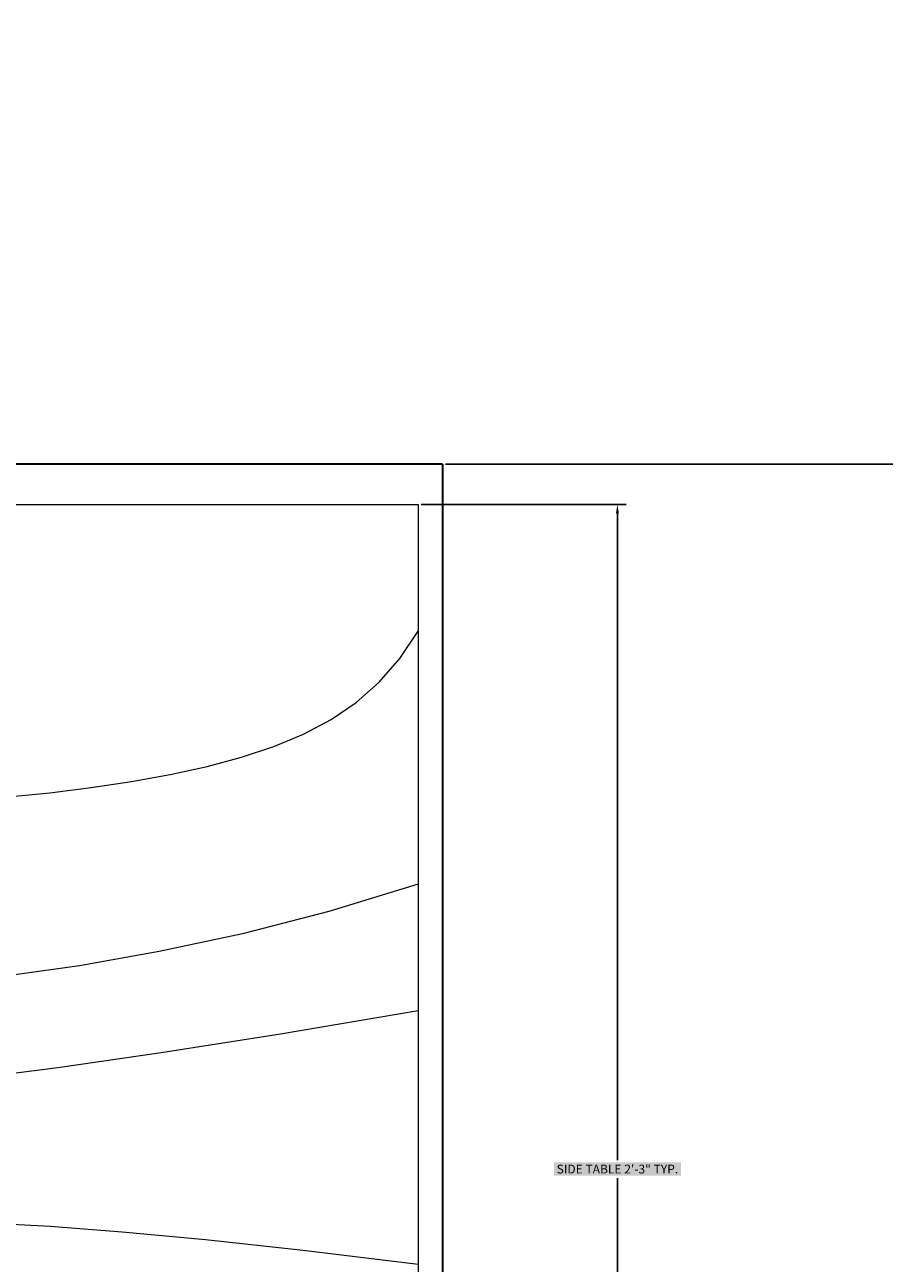
# Model space of a CAD drawing. Units: inches. Extents: x -128 to 854, y -395 to 398.
# Tile 41 of 61: x 296 to 314, y 170 to 196. Entities that reach past the tile are written whole.
import ezdxf

# ---------------------------------------------------------------- set-up
doc = ezdxf.new("R2010")
doc.units = ezdxf.units.IN
doc.header["$MEASUREMENT"] = 0
for name, color, linetype, lineweight in [('A-ANNO-DIMS', 2, 'Continuous', 18), ('A-FURN', 8, 'Continuous', 18), ('A-WALL', 4, 'Continuous', 35)]:
    doc.layers.add(name, color=color, linetype=linetype, lineweight=lineweight)
doc.styles.get("Standard").update_dxf_attribs({"font": 'arial.ttf'})
doc.dimstyles.get("Standard").update_dxf_attribs({"dimtxt": 0.18, "dimasz": 0.18, "dimexe": 0.18, "dimexo": 0.0625, "dimgap": 0.09, "dimtad": 0, "dimtih": 1, "dimtoh": 1, "dimdec": 1, "dimzin": 0, "dimdsep": 46, "dimlunit": 4, "dimtxsty": 'Standard', "dimcen": 0.09, "dimclrd": 1, "dimclre": 2, "dimclrt": 6, "dimadec": 0, "dimazin": 0, "dimtfac": 1, "dimtdec": 1, "dimtofl": 0, "dimtmove": 0, "dimatfit": 3, "dimfxl": 1, "dimtfill": 2, "dimtfillclr": 3, "dimtolj": 1, "dimtzin": 0, "dimarcsym": 0})

# ---------------------------------------------------------------- blocks, each defined once
blk = doc.blocks.new('Table - Square Woodgrain 42 x 42 in.')
for points in [[(0, -42), (0, 0), (42, 0), (42, -42)], [(29.0383, -9.2382), (30.3655, -9.1068), (31.6728, -8.9455), (32.9461, -8.7535), (34.1717, -8.5304), (35.3358, -8.2756), (36.4268, -7.9863), (37.443, -7.6521), (38.3849, -7.2603), (39.253, -6.7986), (40.048, -6.2542), (40.7705, -5.6147), (41.421, -4.8674), (42, -4)], [(42, -12), (39.1784, -12.8621), (36.4519, -13.5654), (33.8246, -14.1294), (31.3004, -14.5731), (28.8832, -14.9161)], [(42, -16), (37.6529, -16.7365), (33.8802, -17.329), (30.6179, -17.7961), (27.8015, -18.1561)], [(0, -24), (3.9243, -23.6805), (7.4766, -23.4138), (10.6891, -23.1954), (13.5943, -23.0205), (16.2247, -22.8847), (18.6125, -22.7832), (20.7903, -22.7116), (22.7903, -22.6651), (24.6563, -22.642), (26.4764, -22.6507), (28.35, -22.7024), (30.3766, -22.8084), (32.6555, -22.98), (35.2861, -23.2283), (38.3678, -23.5645), (42, -24)]]:
    blk.add_lwpolyline(points)
blk = doc.blocks.new('*D55')
at = {"layer": 'A-ANNO-DIMS', "color": 0, "lineweight": -2, "transparency": 16777216}
for p, q in [((304.81, 186.741), (221.092, 186.741)), ((221.272, 181.741), (221.272, 131.873)), ((221.272, 77.741), (221.272, 127.608)), ((304.81, 72.741), (221.092, 72.741))]:
    blk.add_line(p, q, dxfattribs=at)
at = {"layer": 'A-ANNO-DIMS', "color": 0, "transparency": 16777216}
for points in [[(220.439, 181.741), (222.105, 181.741), (221.272, 186.741)], [(220.439, 77.741), (222.105, 77.741), (221.272, 72.741)]]:
    blk.add_solid(points, dxfattribs=at)
at = {"layer": 'Defpoints', "color": 0, "transparency": 16777216}
for p in [(221.272, 186.741), (304.873, 186.741), (304.873, 72.741)]:
    blk.add_point(p, dxfattribs=at)
at = {"layer": 'A-ANNO-DIMS', "color": 0, "transparency": 16777216, "insert": (221.272, 129.741), "char_height": 4, "attachment_point": 5, "bg_fill": 1, "box_fill_scale": 1.25, "bg_fill_color": 3, "bg_fill_transparency": 0}
blk.add_mtext('\\A1;9\'-6"', dxfattribs=at)
blk = doc.blocks.new('*D87')
at = {"layer": 'A-ANNO-DIMS', "color": 2, "lineweight": -2, "transparency": 16777216}
for p, q in [((304.435, 185.918), (308.616, 185.918)), ((304.435, 158.828), (308.616, 158.828))]:
    blk.add_line(p, q, dxfattribs=at)
at = {"layer": 'A-ANNO-DIMS', "color": 1, "lineweight": -2, "transparency": 16777216}
for p, q in [((308.436, 185.738), (308.436, 172.557)), ((308.436, 159.008), (308.436, 172.19))]:
    blk.add_line(p, q, dxfattribs=at)
at = {"layer": 'A-ANNO-DIMS', "color": 1, "transparency": 16777216}
for points in [[(308.406, 185.738), (308.466, 185.738), (308.436, 185.918)], [(308.406, 159.008), (308.466, 159.008), (308.436, 158.828)]]:
    blk.add_solid(points, dxfattribs=at)
at = {"layer": 'Defpoints', "color": 0, "transparency": 16777216}
for p in [(304.372, 185.918), (308.436, 185.918), (304.372, 158.828)]:
    blk.add_point(p, dxfattribs=at)
at = {"layer": 'A-ANNO-DIMS', "color": 6, "transparency": 16777216, "insert": (308.436, 172.373), "char_height": 0.18, "attachment_point": 5, "bg_fill": 1, "box_fill_scale": 1.25, "bg_fill_color": 3, "bg_fill_transparency": 0}
blk.add_mtext('\\A1;SIDE TABLE 2\'-3" TYP.', dxfattribs=at)
blk = doc.blocks.new('*D98')
at = {"layer": 'A-ANNO-DIMS', "color": 2, "lineweight": -2, "transparency": 16777216}
for p, q in [((313.935, 348.741), (351.853, 348.741)), ((313.935, -89.259), (351.853, -89.259))]:
    blk.add_line(p, q, dxfattribs=at)
at = {"layer": 'A-ANNO-DIMS', "color": 1, "lineweight": -2, "transparency": 16777216}
for p, q in [((351.673, 348.561), (351.673, 129.923)), ((351.673, -89.079), (351.673, 129.559))]:
    blk.add_line(p, q, dxfattribs=at)
at = {"layer": 'A-ANNO-DIMS', "color": 1, "transparency": 16777216}
for points in [[(351.643, 348.561), (351.703, 348.561), (351.673, 348.741)], [(351.643, -89.079), (351.703, -89.079), (351.673, -89.259)]]:
    blk.add_solid(points, dxfattribs=at)
at = {"layer": 'Defpoints', "color": 0, "transparency": 16777216}
for p in [(313.873, 348.741), (351.673, 348.741), (313.873, -89.259)]:
    blk.add_point(p, dxfattribs=at)
at = {"layer": 'A-ANNO-DIMS', "color": 6, "transparency": 16777216, "insert": (351.673, 129.741), "char_height": 0.18, "attachment_point": 5, "bg_fill": 1, "box_fill_scale": 1.25, "bg_fill_color": 3, "bg_fill_transparency": 0}
blk.add_mtext('\\A1;36\'-6"', dxfattribs=at)
blk = doc.blocks.new('*D112')
at = {"layer": 'A-ANNO-DIMS', "color": 2, "lineweight": -2, "transparency": 16777216}
for p, q in [((304.935, 186.741), (351.853, 186.741)), ((304.935, 155.741), (351.853, 155.741))]:
    blk.add_line(p, q, dxfattribs=at)
at = {"layer": 'A-ANNO-DIMS', "color": 1, "lineweight": -2, "transparency": 16777216}
for p, q in [((351.673, 186.561), (351.673, 171.421)), ((351.673, 155.921), (351.673, 171.06))]:
    blk.add_line(p, q, dxfattribs=at)
at = {"layer": 'A-ANNO-DIMS', "color": 1, "transparency": 16777216}
for points in [[(351.643, 186.561), (351.703, 186.561), (351.673, 186.741)], [(351.643, 155.921), (351.703, 155.921), (351.673, 155.741)]]:
    blk.add_solid(points, dxfattribs=at)
at = {"layer": 'Defpoints', "color": 0, "transparency": 16777216}
for p in [(304.873, 186.741), (304.873, 155.741), (351.673, 155.741)]:
    blk.add_point(p, dxfattribs=at)
at = {"layer": 'A-ANNO-DIMS', "color": 6, "transparency": 16777216, "insert": (351.673, 171.241), "char_height": 0.18, "attachment_point": 5, "bg_fill": 1, "box_fill_scale": 1.25, "bg_fill_color": 3, "bg_fill_transparency": 0}
blk.add_mtext('\\A1;2\'-7"', dxfattribs=at)

msp = doc.modelspace()

# ---------------------------------------------------------------- linework, layer by layer
at = {"layer": 'A-WALL'}
for q in [(220.42, 186.741), (304.873, 72.741)]:
    msp.add_line((304.873, 186.741), q, dxfattribs=at)

# ---------------------------------------------------------------- block references
at = {"layer": 'A-FURN', "xscale": 0.6449685946951323, "yscale": 0.6449685946951323, "zscale": 0.6449685946951323}
msp.add_blockref('Table - Square Woodgrain 42 x 42 in.', (277.284, 185.917), dxfattribs=at)

# ---------------------------------------------------------------- dimensions: what is measured, and where the dimension line sits
at = {"layer": 'A-ANNO-DIMS'}
for base, p1, p2, override, picture, middle in [((351.673, 348.741), (313.873, -89.259), (313.873, 348.741), {"dimdec": 1, "dimlfac": 1, "dimrnd": 0, "dimzin": 1, "dimdsep": 46, "dimlunit": 4, "dimfrac": 2}, '*D98', (351.673, 129.741)), ((221.272, 186.741), (304.873, 72.741), (304.873, 186.741), {"dimtxt": 4, "dimasz": 5, "dimclrd": 0, "dimclre": 0, "dimclrt": 0}, '*D55', (221.272, 129.741)), ((351.673, 155.741), (304.873, 186.741), (304.873, 155.741), {"dimdec": 1, "dimlfac": 1, "dimrnd": 0, "dimzin": 1, "dimdsep": 46, "dimlunit": 4, "dimfrac": 2}, '*D112', (351.673, 171.241))]:
    dim = msp.add_linear_dim(base=base, p1=p1, p2=p2, angle=90, dimstyle='Standard', override=override, dxfattribs=at)
    dim.commit()
    dim.dimension.update_dxf_attribs({"geometry": picture, "text_midpoint": middle})
dim = msp.add_linear_dim(base=(308.436, 185.918), p1=(304.372, 158.828), p2=(304.372, 185.918), angle=90, text='SIDE TABLE <> TYP.', dimstyle='Standard', override={"dimdec": 1, "dimlfac": 1, "dimrnd": 0, "dimzin": 1, "dimdsep": 46, "dimlunit": 4, "dimfrac": 2}, dxfattribs=at)
dim.commit()
dim.dimension.update_dxf_attribs({"geometry": '*D87', "text_midpoint": (308.436, 172.373)})

doc.saveas('drawing.dxf')
